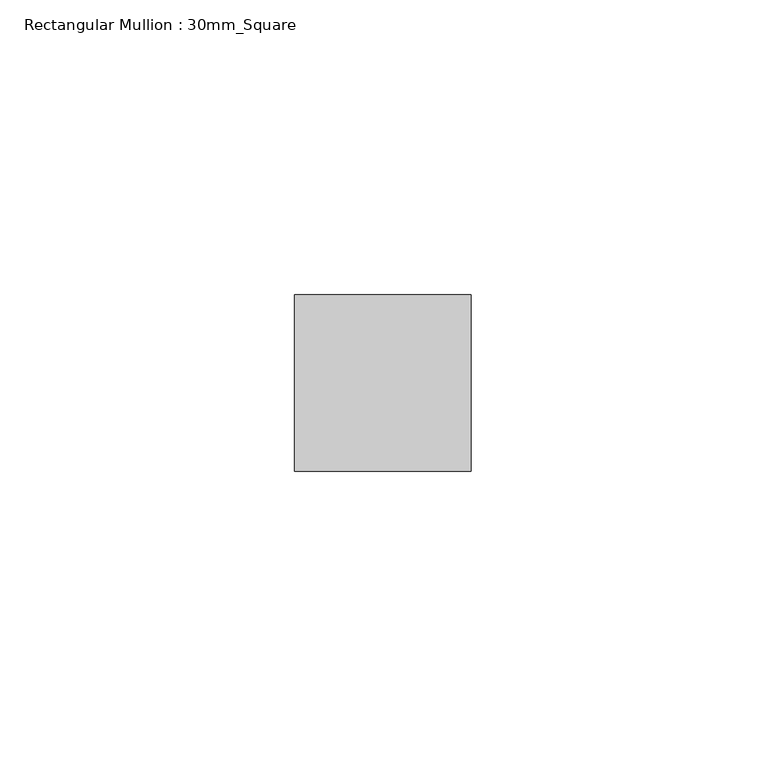
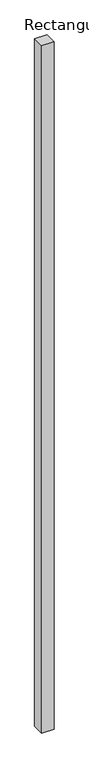
"""IFC4 building model written with IfcOpenShell, lengths in millimetres: member geometry, Rectangular Mullion : 30mm_Square."""

from ifc_helpers import new_model, si_unit, frame, origin, place, context, project, spatial, polyline, outline, extrude, source, transform, mapped, element, save


def rectangular_mullion_30mm_square_b78902bc(model_context):
    return source(origin(), model_context, "Body", "SweptSolid", [
        extrude(outline(polyline([(0.0, 15.0), (0.0, -15.0), (-30.0, -15.0), (-30.0, 15.0), (0.0, 15.0)])), frame((0.0, 0.0, -1785.0000003), z_axis=(0.0, 0.0, 1.0), x_axis=(1.0, 0.0, 0.0)), (0.0, 0.0, 1.0), 1785.0000003),
    ])


if __name__ == "__main__":
    model = new_model("IFC4")
    model_context = context("Model", 3, world=origin())
    ifc_project = project(units=[si_unit("LENGTHUNIT", "METRE", prefix="MILLI")], contexts=[model_context])
    site = spatial("IfcSite", under=ifc_project)
    building = spatial("IfcBuilding", under=site)
    placement = place(None, origin())
    rectangular_mullion_30mm_square_shape = rectangular_mullion_30mm_square_b78902bc(model_context)
    element("IfcMember", 1, ObjectType="Rectangular Mullion : 30mm_Square", at=placement, inside=building, context=model_context, shape_type="MappedRepresentation", body=[
        mapped(rectangular_mullion_30mm_square_shape, transform((0.0, 0.0, 0.0), x_axis=(1.0, 0.0, 0.0), y_axis=(0.0, 1.0, 0.0), z_axis=(0.0, 0.0, 1.0))),
    ])
    save(model, "model.ifc")

# Revit data of these elements
# Type "Rectangular Mullion : 30mm_Square"
#   Keynote = "H11"
#   built-in parameter 1007304 = 0.0984252 (stored number, unit not read)
#   built-in parameter 1007301 = 0.0492126 (stored number, unit not read)
#   built-in parameter 1007300 = 0.0492126 (stored number, unit not read)
# Element 1 (IfcMember, "Rectangular Mullion : 30mm_Square")
#   Materials on its faces: "Aluminium"
# Materials
#   "Aluminium": class "Metal", colour RGB 247 247 247, transparency 0, Description = "Aluminium 6061", Cost = 0
